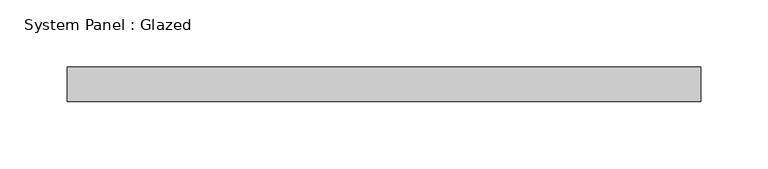
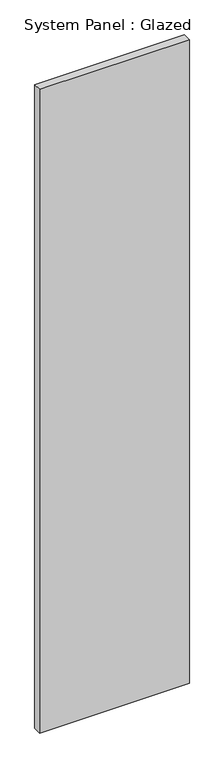
"""IFC4 building model written with IfcOpenShell, lengths in millimetres: plate geometry, System Panel : Glazed."""

from ifc_helpers import new_model, si_unit, origin, origin_with_axes, place, context, project, spatial, polyline, outline, extrude, source, transform, mapped, element, save


def system_panel_glazed_d35b251a(model_context):
    return source(origin(), model_context, "Body", "SweptSolid", [
        extrude(outline(polyline([(234.95, 19.05), (-234.95, 19.05), (-234.95, 44.45), (234.95, 44.45), (234.95, 19.05)])), origin_with_axes(), (0.0, 0.0, 1.0), 2133.6),
    ])


if __name__ == "__main__":
    model = new_model("IFC4")
    model_context = context("Model", 3, world=origin())
    ifc_project = project(units=[si_unit("LENGTHUNIT", "METRE", prefix="MILLI")], contexts=[model_context])
    site = spatial("IfcSite", under=ifc_project)
    building = spatial("IfcBuilding", under=site)
    placement = place(None, origin())
    system_panel_glazed_shape = system_panel_glazed_d35b251a(model_context)
    element("IfcPlate", 1, ObjectType="System Panel : Glazed", at=placement, inside=building, context=model_context, shape_type="MappedRepresentation", body=[
        mapped(system_panel_glazed_shape, transform((0.0, 0.0, 0.0), x_axis=(1.0, 0.0, 0.0), y_axis=(0.0, 1.0, 0.0), z_axis=(0.0, 0.0, 1.0))),
    ])
    save(model, "model.ifc")

# Revit data of these elements
# Type "System Panel : Glazed"
#   Construction Type Id = "GSP4R"
#   Analytic Construction = "1/8 in Pilkington single glazing"
#   Visual Light Transmittance = 0.9
#   Solar Heat Gain Coefficient = 0.86
#   Heat Transfer Coefficient (U) = 1.18115 BTU/(h·ft²·°F)
#   Define Thermal Properties by = 1
# Element 1 (IfcPlate, "System Panel : Glazed")
#   Materials on its faces: "Glass"
# Materials
#   "Glass": class "Glass", colour RGB 0 128 192, transparency 0.75, Description = "Soda Lime Glass", Cost = 0
